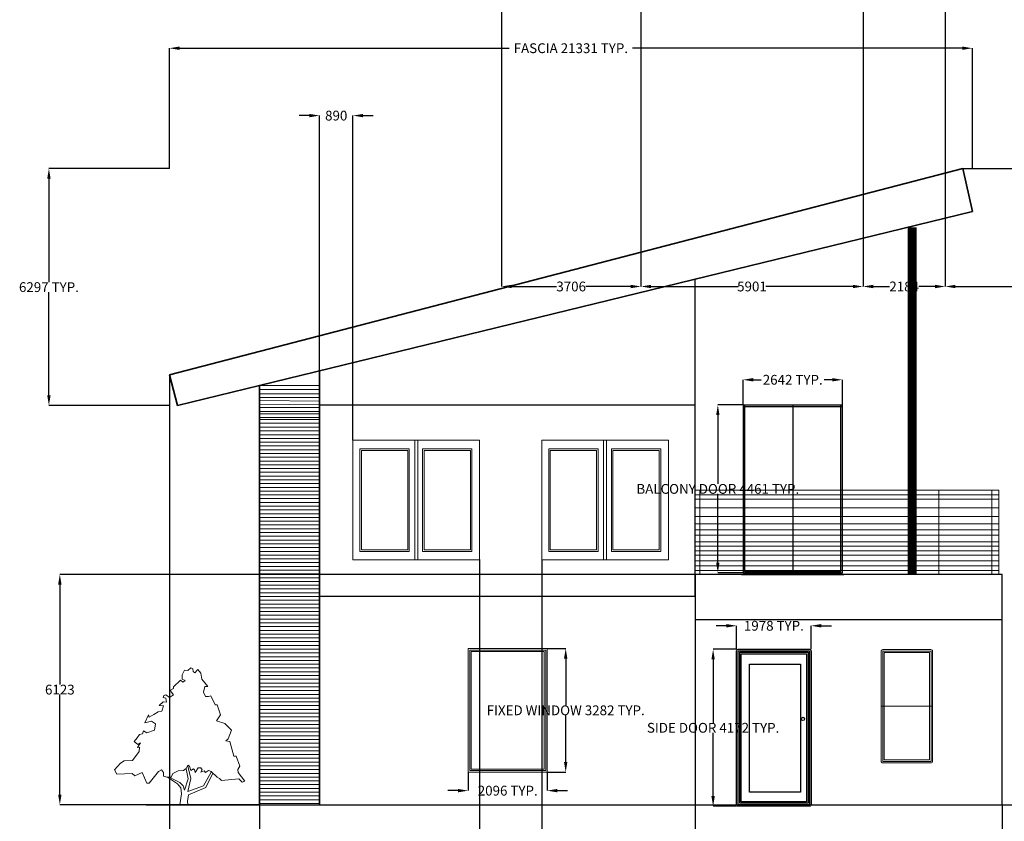
# Model space of a CAD drawing. Units: millimetres. Extents: x 23 to 3809233, y 4 to 290343.
# Tile 4 of 8: x 1889493 to 1915648, y 151826 to 173128. Entities that reach past the tile are written whole.
import ezdxf

# ---------------------------------------------------------------- set-up
doc = ezdxf.new("R2010")
doc.units = ezdxf.units.MM
doc.header["$MEASUREMENT"] = 0
for name, color, linetype, lineweight in [('A-ANNO-DIMS', 2, 'Continuous', 18), ('A-COLS', 7, 'Continuous', 35), ('A-DOOR', 3, 'Continuous', 25), ('A-ELEV', 7, 'Continuous', 25), ('A-ELEV-GRND', 7, 'Continuous', 30), ('A-FLOR-RAIL', 8, 'Continuous', 18), ('A-GLAZ', 4, 'Continuous', 18), ('A-ROOF', 7, 'Continuous', 35), ('A-WALL-PATT', 252, 'Continuous', 13), ('L-PLNT', 94, 'Continuous', 13)]:
    doc.layers.add(name, color=color, linetype=linetype, lineweight=lineweight)
doc.styles.get("Standard").update_dxf_attribs({"font": 'arial.ttf'})
doc.dimstyles.get("Standard").update_dxf_attribs({"dimtxt": 260.18, "dimasz": 270.18, "dimexe": 0.18, "dimexo": 0.0625, "dimgap": 0.09, "dimtad": 0, "dimtih": 1, "dimtoh": 1, "dimdec": 0, "dimzin": 0, "dimdsep": 46, "dimtxsty": 'Standard', "dimcen": 0.09, "dimadec": 0, "dimazin": 0, "dimtfac": 1, "dimtdec": 0, "dimtofl": 0, "dimtmove": 0, "dimatfit": 3, "dimfxl": 1, "dimtolj": 1, "dimtzin": 0, "dimarcsym": 0})

# ---------------------------------------------------------------- blocks, each defined once
blk = doc.blocks.new('*U4')
for points in [[(22.0124, 137.721), (18.5475, 141.5624), (15.5282, 138.2446), (13.8028, 139.3505), (13.3714, 142.1153), (11.2148, 143.2214), (8.1954, 140.4564), (4.7447, 141.0094), (2.1567, 136.0326), (2.1567, 131.6088), (5.6074, 129.9499), (3.0193, 128.2909), (0.4313, 130.5029), (-6.9015, 123.3141), (-6.9015, 121.6552), (-9.9208, 119.9963), (-9.0581, 118.3373), (-6.9015, 115.0195), (-10.7835, 112.2546), (-14.6656, 115.0195), (-16.8222, 114.4665), (-17.6849, 112.2546), (-14.6656, 111.7016), (-14.2342, 107.2778), (-17.6065, 107.8307), (-21.5669, 103.9599), (-17.2536, 103.4069), (-18.9789, 97.8771), (-22.8609, 97.3241), (-27.1743, 94.5593), (-32.3504, 91.7944), (-32.7817, 94.0063), (-36.6638, 85.7116), (-29.7624, 87.3705), (-25.449, 84.6056), (-26.743, 77.9699), (-34.507, 75.205), (-37.9578, 77.4169), (-39.2518, 74.099), (-42.2711, 73.5461), (-44.8592, 70.2282), (-47.8786, 66.3574), (-43.9965, 63.0395), (-41.4085, 64.6985), (-44.3346, 59.8898), (-42.2089, 60.1377), (-42.5159, 55.7849), (-49.6039, 46.4502), (-58.2307, 45.8972), (-62.1127, 43.6853), (-68.5828, 36.4966), (-65.9947, 32.0727), (-50.0352, 32.6257), (-47.0159, 30.4138), (-39.6831, 33.7317), (-34.507, 22.6721), (-32.3504, 22.6721), (-22.4296, 34.8376), (-19.4102, 36.4966), (-17.2536, 33.7317), (-17.2536, 29.8608), (-13.8028, 28.7549), (-9.0581, 28.7549), (-7.3328, 32.6257), (-1.7254, 35.3906), (3.8821, 35.9436), (6.4701, 38.1555), (6.9014, 38.7085), (8.1954, 41.4734), (9.9208, 40.3674), (11.2148, 35.9436), (14.2341, 37.6025), (15.0968, 36.4966), (15.9595, 33.7317), (18.9789, 38.7085), (21.9982, 38.7085), (23.2922, 36.4966), (21.9982, 34.2847), (25.4489, 35.3906), (26.743, 33.7317), (29.7623, 35.9436), (32.7817, 34.8376), (38.8204, 28.7549), (41.4084, 27.6489), (43.5651, 25.437), (61.6813, 27.0959), (65.132, 23.7781), (67.7201, 24.884), (60.8186, 33.7317), (60.3873, 37.0495), (62.544, 40.3674), (58.662, 50.874), (56.5053, 50.874), (52.1919, 66.3574), (47.8785, 66.9103), (50.4665, 69.1222), (53.9172, 77.9699), (47.0158, 85.1586), (38.3891, 87.9235), (42.2711, 94.0063)], [(42.2711, 94.0063), (38.8204, 104.5129), (36.6637, 104.5129), (32.3503, 113.9135), (29.7623, 113.3605), (26.743, 113.3605), (24.5862, 117.7844), (25.8802, 123.8671), (29.331, 123.8671), (22.8609, 131.6088), (21.9982, 137.6916)], [(-9.9208, 28.2019), (0, 23.2251), (3.4507, 19.9072), (4.7447, 15.4834), (8.6267, 27.0959), (6.4701, 37.6025)], [(34.5071, 33.1787), (27.1743, 18.2483), (9.0581, 10.5066), (7.7641, 3.8708), (8.1954, 0)], [(8.1954, 40.3674), (11.2148, 27.6489), (8.1954, 13.8245), (24.5862, 19.9072), (32.7817, 34.2847)], [(-12.9401, 28.7549), (-2.588, 22.1191), (0.8626, 17.6953), (1.7253, 11.6125), (0, 0)]]:
    blk.add_lwpolyline(points)
blk = doc.blocks.new('SIDE-ENTRY-DOOR-ELEV')
for points in [[(0, 4129, -0.414214), (43, 4172), (1935, 4172, -0.414214), (1978, 4129), (1978, 43, -0.414214), (1935, 0), (43, 0, -0.414214), (0, 43)], [(40, 4129, -0.414214), (43, 4132), (1935, 4132, -0.414214), (1938, 4129), (1938, 43, -0.414214), (1935, 40), (43, 40, -0.414214), (40, 43)], [(337, 3772, -0.414214), (340, 3775), (1691, 3775, -0.414214), (1694, 3772), (1694, 380, -0.414214), (1691, 377), (340, 377, -0.414214), (337, 380)]]:
    blk.add_lwpolyline(points, format="xyb", close=True)
for points in [[(80, 4092), (1898, 4092), (1898, 80), (80, 80)], [(120, 4052), (1858, 4052), (1858, 120), (120, 120)]]:
    blk.add_lwpolyline(points, close=True)
blk.add_circle((1762, 2322), 43.3)
blk = doc.blocks.new('FIXED-WINDOW-ELEV')
blk.add_lwpolyline([(0, 3279, -0.414214), (3, 3282), (2093, 3282, -0.414214), (2096, 3279), (2096, 3, -0.414214), (2093, 0), (3, 0, -0.414214), (0, 3)], format="xyb", close=True)
for points in [[(40, 3242), (2056, 3242), (2056, 40), (40, 40)], [(80, 3202), (2016, 3202), (2016, 80), (80, 80)]]:
    blk.add_lwpolyline(points, close=True)
blk = doc.blocks.new('TRANSOM-WINDOW-ELEV')
blk.add_line((0, 1506), (1365, 1506))
for points in [[(0, 2969, -0.414214), (43, 3012), (1322, 3012, -0.414214), (1365, 2969), (1365, 43, -0.414214), (1322, 0), (43, 0, -0.414214), (0, 43)], [(40, 2969, -0.414214), (43, 2972), (1322, 2972, -0.414214), (1325, 2969), (1325, 43, -0.414214), (1322, 40), (43, 40, -0.414214), (40, 43)]]:
    blk.add_lwpolyline(points, format="xyb", close=True)
blk.add_lwpolyline([(80, 2932), (1285, 2932), (1285, 80), (80, 80)], close=True)
blk = doc.blocks.new('BALCONY-GUARD-ELEV')
for p, q in [((8065, 2239), (0, 2239)), ((0, 2109), (8065, 2109)), ((129, 2239), (129, 0)), ((6472, 2239), (6472, 0)), ((7879, 2239), (7879, 0)), ((8065, 0), (8065, 2239)), ((0, 1995), (8065, 1995)), ((0, 1772), (8065, 1772)), ((0, 1540), (8065, 1540)), ((0, 1341), (8065, 1341)), ((0, 1187), (8065, 1187)), ((0, 1045), (8065, 1045)), ((0, 866), (8065, 866)), ((0, 745), (8065, 745)), ((0, 622), (8065, 622)), ((0, 507), (8065, 507)), ((0, 360), (8065, 360)), ((8065, 360), (8065, 360)), ((0, 225), (8065, 225)), ((0, 103), (8065, 103))]:
    blk.add_line(p, q)
blk = doc.blocks.new('ROOF-FASCIA-SIDE-ELEV')
for p, q in [((21076, 6297), (0, 817)), ((21331, 5154), (21076, 6297)), ((2399, 534), (21331, 5154)), ((0, 817), (212, 0)), ((2399, 534), (212, 0))]:
    blk.add_line(p, q)
blk = doc.blocks.new('BALCONY-SUPPORT-ELEV')
for p, q in [((0, 0), (0, 9216)), ((40, 0), (40, 9216)), ((80, 0), (80, 9216)), ((120, 0), (120, 9216)), ((120, 0), (120, 9216)), ((160, 0), (160, 9216)), ((200, 0), (200, 9216))]:
    blk.add_line(p, q)
blk = doc.blocks.new('BALCONY-GLAZED-DOOR-ELEV')
for p, q in [((0, 4461), (2642, 4461)), ((1321, 4461), (1321, 0)), ((0, 4421), (2642, 4421))]:
    blk.add_line(p, q)
for points in [[(0, 4461), (0, 0), (2642, 0), (2642, 4461)], [(40, 4461), (40, 40), (2602, 40), (2602, 4461)]]:
    blk.add_lwpolyline(points)
blk = doc.blocks.new('*D28')
at = {"layer": 'A-ANNO-DIMS', "color": 0, "lineweight": -2, "transparency": 16777216}
for p, q in [((1893468, 169170), (1893468, 172370)), ((1893739, 172370), (1902498, 172370)), ((1914529, 172370), (1905770, 172370)), ((1914799, 169170), (1914799, 172370))]:
    blk.add_line(p, q, dxfattribs=at)
at = {"layer": 'A-ANNO-DIMS', "color": 0, "transparency": 16777216}
for points in [[(1893739, 172415), (1893739, 172325), (1893468, 172370)], [(1914529, 172415), (1914529, 172325), (1914799, 172370)]]:
    blk.add_solid(points, dxfattribs=at)
at = {"layer": 'Defpoints', "color": 0, "transparency": 16777216}
for p in [(1914799, 172370), (1893468, 169170), (1914799, 169170)]:
    blk.add_point(p, dxfattribs=at)
at = {"layer": 'A-ANNO-DIMS', "color": 0, "transparency": 16777216, "insert": (1904134, 172370), "char_height": 260.18, "attachment_point": 5}
blk.add_mtext('\\A1;FASCIA 21331 TYP.', dxfattribs=at)
blk = doc.blocks.new('*D29')
at = {"layer": 'A-ANNO-DIMS', "color": 0, "lineweight": -2, "transparency": 16777216}
for p, q in [((1893468, 169170), (1890268, 169170)), ((1890269, 168900), (1890269, 166154)), ((1890269, 163143), (1890269, 165889)), ((1893468, 162873), (1890268, 162873))]:
    blk.add_line(p, q, dxfattribs=at)
at = {"layer": 'A-ANNO-DIMS', "color": 0, "transparency": 16777216}
for points in [[(1890224, 168900), (1890314, 168900), (1890269, 169170)], [(1890224, 163143), (1890314, 163143), (1890269, 162873)]]:
    blk.add_solid(points, dxfattribs=at)
at = {"layer": 'Defpoints', "color": 0, "transparency": 16777216}
for p in [(1890269, 169170), (1893468, 169170), (1893468, 162873)]:
    blk.add_point(p, dxfattribs=at)
at = {"layer": 'A-ANNO-DIMS', "color": 0, "transparency": 16777216, "insert": (1890269, 166021), "char_height": 260.18, "attachment_point": 5}
blk.add_mtext('\\A1;6297 TYP.', dxfattribs=at)
blk = doc.blocks.new('*D32')
at = {"layer": 'A-ANNO-DIMS', "color": 0, "lineweight": -2, "transparency": 16777216}
for p, q in [((1908707, 162890), (1908038, 162890)), ((1908038, 162620), (1908038, 160794)), ((1908038, 158699), (1908038, 160524)), ((1908707, 158429), (1908038, 158429))]:
    blk.add_line(p, q, dxfattribs=at)
at = {"layer": 'A-ANNO-DIMS', "color": 0, "transparency": 16777216}
for points in [[(1907993, 162620), (1908083, 162620), (1908038, 162890)], [(1907993, 158699), (1908083, 158699), (1908038, 158429)]]:
    blk.add_solid(points, dxfattribs=at)
at = {"layer": 'Defpoints', "color": 0, "transparency": 16777216}
for p in [(1908038, 162890), (1908707, 162890), (1908707, 158429)]:
    blk.add_point(p, dxfattribs=at)
at = {"layer": 'A-ANNO-DIMS', "color": 0, "transparency": 16777216, "insert": (1908038, 160659), "char_height": 260.18, "attachment_point": 5}
blk.add_mtext('\\A1;BALCONY DOOR 4461 TYP.', dxfattribs=at)
blk = doc.blocks.new('*D33')
at = {"layer": 'A-ANNO-DIMS', "color": 0, "lineweight": -2, "transparency": 16777216}
for p, q in [((1908707, 162890), (1908707, 163559)), ((1908977, 163559), (1909190, 163559)), ((1911079, 163559), (1910866, 163559)), ((1911349, 162890), (1911349, 163559))]:
    blk.add_line(p, q, dxfattribs=at)
at = {"layer": 'A-ANNO-DIMS', "color": 0, "transparency": 16777216}
for points in [[(1908977, 163604), (1908977, 163514), (1908707, 163559)], [(1911079, 163604), (1911079, 163514), (1911349, 163559)]]:
    blk.add_solid(points, dxfattribs=at)
at = {"layer": 'Defpoints', "color": 0, "transparency": 16777216}
for p in [(1911349, 163559), (1908707, 162890), (1911349, 162890)]:
    blk.add_point(p, dxfattribs=at)
at = {"layer": 'A-ANNO-DIMS', "color": 0, "transparency": 16777216, "insert": (1910028, 163559), "char_height": 260.18, "attachment_point": 5}
blk.add_mtext('\\A1;2642 TYP.', dxfattribs=at)
blk = doc.blocks.new('*D34')
at = {"layer": 'A-ANNO-DIMS', "color": 0, "lineweight": -2, "transparency": 16777216}
for p, q in [((1908538, 156397), (1907912, 156397)), ((1907913, 156126), (1907913, 154445)), ((1907913, 152495), (1907913, 154176)), ((1908538, 152225), (1907912, 152225))]:
    blk.add_line(p, q, dxfattribs=at)
at = {"layer": 'A-ANNO-DIMS', "color": 0, "transparency": 16777216}
for points in [[(1907868, 156126), (1907958, 156126), (1907913, 156397)], [(1907868, 152495), (1907958, 152495), (1907913, 152225)]]:
    blk.add_solid(points, dxfattribs=at)
at = {"layer": 'Defpoints', "color": 0, "transparency": 16777216}
for p in [(1907913, 156397), (1908538, 156397), (1908538, 152225)]:
    blk.add_point(p, dxfattribs=at)
at = {"layer": 'A-ANNO-DIMS', "color": 0, "transparency": 16777216, "insert": (1907913, 154311), "char_height": 260.18, "attachment_point": 5}
blk.add_mtext('\\A1;SIDE DOOR 4172 TYP.', dxfattribs=at)
blk = doc.blocks.new('*D35')
at = {"layer": 'A-ANNO-DIMS', "color": 0, "lineweight": -2, "transparency": 16777216}
for p, q in [((1908268, 157022), (1907998, 157022)), ((1908538, 156397), (1908538, 157023)), ((1910516, 156397), (1910516, 157023)), ((1910786, 157022), (1911056, 157022))]:
    blk.add_line(p, q, dxfattribs=at)
at = {"layer": 'A-ANNO-DIMS', "color": 0, "transparency": 16777216}
for points in [[(1908268, 157067), (1908268, 156977), (1908538, 157022)], [(1910786, 157067), (1910786, 156977), (1910516, 157022)]]:
    blk.add_solid(points, dxfattribs=at)
at = {"layer": 'Defpoints', "color": 0, "transparency": 16777216}
for p in [(1910516, 157022), (1908538, 156397), (1910516, 156397)]:
    blk.add_point(p, dxfattribs=at)
at = {"layer": 'A-ANNO-DIMS', "color": 0, "transparency": 16777216, "insert": (1909527, 157022), "char_height": 260.18, "attachment_point": 5}
blk.add_mtext('\\A1;1978 TYP.', dxfattribs=at)
blk = doc.blocks.new('*D36')
at = {"layer": 'A-ANNO-DIMS', "color": 0, "lineweight": -2, "transparency": 16777216}
for p, q in [((1903505, 156416), (1903997, 156416)), ((1903997, 156146), (1903997, 154910)), ((1903997, 153404), (1903997, 154640)), ((1903505, 153134), (1903997, 153134))]:
    blk.add_line(p, q, dxfattribs=at)
at = {"layer": 'A-ANNO-DIMS', "color": 0, "transparency": 16777216}
for points in [[(1903952, 156146), (1904042, 156146), (1903997, 156416)], [(1903952, 153404), (1904042, 153404), (1903997, 153134)]]:
    blk.add_solid(points, dxfattribs=at)
at = {"layer": 'Defpoints', "color": 0, "transparency": 16777216}
for p in [(1903505, 156416), (1903997, 156416), (1903505, 153134)]:
    blk.add_point(p, dxfattribs=at)
at = {"layer": 'A-ANNO-DIMS', "color": 0, "transparency": 16777216, "insert": (1903997, 154775), "char_height": 260.18, "attachment_point": 5}
blk.add_mtext('\\A1;FIXED WINDOW 3282 TYP.', dxfattribs=at)
blk = doc.blocks.new('*D37')
at = {"layer": 'A-ANNO-DIMS', "color": 0, "lineweight": -2, "transparency": 16777216}
for p, q in [((1901409, 153134), (1901409, 152641)), ((1903505, 153134), (1903505, 152641)), ((1901139, 152641), (1900869, 152641)), ((1903775, 152641), (1904045, 152641))]:
    blk.add_line(p, q, dxfattribs=at)
at = {"layer": 'A-ANNO-DIMS', "color": 0, "transparency": 16777216}
for points in [[(1901139, 152686), (1901139, 152596), (1901409, 152641)], [(1903775, 152686), (1903775, 152596), (1903505, 152641)]]:
    blk.add_solid(points, dxfattribs=at)
at = {"layer": 'Defpoints', "color": 0, "transparency": 16777216}
for p in [(1901409, 153134), (1903505, 153134), (1903505, 152641)]:
    blk.add_point(p, dxfattribs=at)
at = {"layer": 'A-ANNO-DIMS', "color": 0, "transparency": 16777216, "insert": (1902457, 152641), "char_height": 260.18, "attachment_point": 5}
blk.add_mtext('\\A1;2096 TYP.', dxfattribs=at)
blk = doc.blocks.new('*D80')
at = {"layer": 'A-ANNO-DIMS', "color": 0, "lineweight": -2, "transparency": 16777216}
for p, q in [((1893468, 163690), (1893468, 149029)), ((1915588, 152264), (1915588, 149029)), ((1893739, 149029), (1904037, 149029)), ((1915318, 149029), (1905020, 149029))]:
    blk.add_line(p, q, dxfattribs=at)
at = {"layer": 'A-ANNO-DIMS', "color": 0, "transparency": 16777216}
for points in [[(1893739, 149074), (1893739, 148984), (1893468, 149029)], [(1915318, 149074), (1915318, 148984), (1915588, 149029)]]:
    blk.add_solid(points, dxfattribs=at)
at = {"layer": 'Defpoints', "color": 0, "transparency": 16777216}
for p in [(1893468, 163690), (1915588, 152265), (1915588, 149029)]:
    blk.add_point(p, dxfattribs=at)
at = {"layer": 'A-ANNO-DIMS', "color": 0, "transparency": 16777216, "insert": (1904528, 149029), "char_height": 260.2, "attachment_point": 5}
blk.add_mtext('\\A1;22120', dxfattribs=at)
blk = doc.blocks.new('*D81')
at = {"layer": 'A-ANNO-DIMS', "color": 0, "lineweight": -2, "transparency": 16777216}
for p, q in [((1914545, 169170), (1921388, 169170)), ((1921387, 168900), (1921387, 160850)), ((1921387, 152535), (1921387, 160584)), ((1915588, 152265), (1921388, 152265))]:
    blk.add_line(p, q, dxfattribs=at)
at = {"layer": 'A-ANNO-DIMS', "color": 0, "transparency": 16777216}
for points in [[(1921342, 168900), (1921433, 168900), (1921387, 169170)], [(1921342, 152535), (1921433, 152535), (1921387, 152265)]]:
    blk.add_solid(points, dxfattribs=at)
at = {"layer": 'Defpoints', "color": 0, "transparency": 16777216}
for p in [(1914545, 169170), (1921387, 169170), (1915588, 152265)]:
    blk.add_point(p, dxfattribs=at)
at = {"layer": 'A-ANNO-DIMS', "color": 0, "transparency": 16777216, "insert": (1921387, 160717), "char_height": 260.2, "attachment_point": 5}
blk.add_mtext('\\A1;16905', dxfattribs=at)
blk = doc.blocks.new('*D82')
at = {"layer": 'A-ANNO-DIMS', "color": 0, "lineweight": -2, "transparency": 16777216}
for p, q in [((1895867, 152264), (1895867, 149029)), ((1907434, 152264), (1907434, 149029)), ((1896137, 149029), (1901173, 149029)), ((1907164, 149029), (1902128, 149029))]:
    blk.add_line(p, q, dxfattribs=at)
at = {"layer": 'A-ANNO-DIMS', "color": 0, "transparency": 16777216}
for points in [[(1896137, 149074), (1896137, 148984), (1895867, 149029)], [(1907164, 149074), (1907164, 148984), (1907434, 149029)]]:
    blk.add_solid(points, dxfattribs=at)
at = {"layer": 'Defpoints', "color": 0, "transparency": 16777216}
for p in [(1895867, 152265), (1907434, 152265), (1907434, 149029)]:
    blk.add_point(p, dxfattribs=at)
at = {"layer": 'A-ANNO-DIMS', "color": 0, "transparency": 16777216, "insert": (1901651, 149029), "char_height": 260.2, "attachment_point": 5}
blk.add_mtext('\\A1;11567', dxfattribs=at)
blk = doc.blocks.new('*D83')
at = {"layer": 'A-ANNO-DIMS', "color": 0, "lineweight": -2, "transparency": 16777216}
for p, q in [((1907435, 158388), (1890558, 158388)), ((1890559, 158117), (1890559, 155459)), ((1890559, 152535), (1890559, 155193)), ((1895867, 152265), (1890558, 152265))]:
    blk.add_line(p, q, dxfattribs=at)
at = {"layer": 'A-ANNO-DIMS', "color": 0, "transparency": 16777216}
for points in [[(1890514, 158117), (1890604, 158117), (1890559, 158388)], [(1890514, 152535), (1890604, 152535), (1890559, 152265)]]:
    blk.add_solid(points, dxfattribs=at)
at = {"layer": 'Defpoints', "color": 0, "transparency": 16777216}
for p in [(1890559, 158388), (1907435, 158388), (1895867, 152265)]:
    blk.add_point(p, dxfattribs=at)
at = {"layer": 'A-ANNO-DIMS', "color": 0, "transparency": 16777216, "insert": (1890559, 155326), "char_height": 260.2, "attachment_point": 5}
blk.add_mtext('\\A1;6123', dxfattribs=at)
blk = doc.blocks.new('*D84')
at = {"layer": 'A-ANNO-DIMS', "color": 0, "lineweight": -2, "transparency": 16777216}
for p, q in [((1897185, 170579), (1896915, 170579)), ((1897456, 162891), (1897456, 170580)), ((1898346, 161958), (1898346, 170580)), ((1898616, 170579), (1898886, 170579))]:
    blk.add_line(p, q, dxfattribs=at)
at = {"layer": 'A-ANNO-DIMS', "color": 0, "transparency": 16777216}
for points in [[(1897185, 170624), (1897185, 170534), (1897456, 170579)], [(1898616, 170624), (1898616, 170534), (1898346, 170579)]]:
    blk.add_solid(points, dxfattribs=at)
at = {"layer": 'Defpoints', "color": 0, "transparency": 16777216}
for p in [(1898346, 170579), (1897456, 162891), (1898346, 161958)]:
    blk.add_point(p, dxfattribs=at)
at = {"layer": 'A-ANNO-DIMS', "color": 0, "transparency": 16777216, "insert": (1897901, 170579), "char_height": 260.2, "attachment_point": 5}
blk.add_mtext('\\A1;890', dxfattribs=at)
blk = doc.blocks.new('*D85')
at = {"layer": 'A-ANNO-DIMS', "color": 0, "lineweight": -2, "transparency": 16777216}
for p, q in [((1901710, 158781), (1901710, 149029)), ((1903361, 158781), (1903361, 149029)), ((1901980, 149029), (1902184, 149029)), ((1903091, 149029), (1902887, 149029))]:
    blk.add_line(p, q, dxfattribs=at)
at = {"layer": 'A-ANNO-DIMS', "color": 0, "transparency": 16777216}
for points in [[(1901980, 149074), (1901980, 148984), (1901710, 149029)], [(1903091, 149074), (1903091, 148984), (1903361, 149029)]]:
    blk.add_solid(points, dxfattribs=at)
at = {"layer": 'Defpoints', "color": 0, "transparency": 16777216}
for p in [(1901710, 158781), (1903361, 158781), (1903361, 149029)]:
    blk.add_point(p, dxfattribs=at)
at = {"layer": 'A-ANNO-DIMS', "color": 0, "transparency": 16777216, "insert": (1902536, 149029), "char_height": 260.2, "attachment_point": 5}
blk.add_mtext('\\A1;1651', dxfattribs=at)
blk = doc.blocks.new('*D96')
at = {"layer": 'A-ANNO-DIMS', "color": 0, "lineweight": -2, "transparency": 16777216}
for p, q in [((1902289, 175032), (1902289, 166038)), ((1905995, 175031), (1905995, 166038)), ((1902560, 166038), (1903754, 166038)), ((1905725, 166038), (1904531, 166038))]:
    blk.add_line(p, q, dxfattribs=at)
at = {"layer": 'A-ANNO-DIMS', "color": 0, "transparency": 16777216}
for points in [[(1902560, 166083), (1902560, 165993), (1902289, 166038)], [(1905725, 166083), (1905725, 165993), (1905995, 166038)]]:
    blk.add_solid(points, dxfattribs=at)
at = {"layer": 'Defpoints', "color": 0, "transparency": 16777216}
for p in [(1902289, 175032), (1905995, 175031), (1905995, 166038)]:
    blk.add_point(p, dxfattribs=at)
at = {"layer": 'A-ANNO-DIMS', "color": 0, "transparency": 16777216, "insert": (1904142, 166038), "char_height": 260.2, "attachment_point": 5}
blk.add_mtext('\\A1;3706', dxfattribs=at)
blk = doc.blocks.new('*D97')
at = {"layer": 'A-ANNO-DIMS', "color": 0, "lineweight": -2, "transparency": 16777216}
for p, q in [((1905995, 175031), (1905995, 166038)), ((1911896, 175048), (1911896, 166038)), ((1906265, 166038), (1908582, 166038)), ((1911626, 166038), (1909309, 166038))]:
    blk.add_line(p, q, dxfattribs=at)
at = {"layer": 'A-ANNO-DIMS', "color": 0, "transparency": 16777216}
for points in [[(1906265, 166083), (1906265, 165993), (1905995, 166038)], [(1911626, 166083), (1911626, 165993), (1911896, 166038)]]:
    blk.add_solid(points, dxfattribs=at)
at = {"layer": 'Defpoints', "color": 0, "transparency": 16777216}
for p in [(1905995, 175031), (1911896, 175048), (1911896, 166038)]:
    blk.add_point(p, dxfattribs=at)
at = {"layer": 'A-ANNO-DIMS', "color": 0, "transparency": 16777216, "insert": (1908945, 166038), "char_height": 260.2, "attachment_point": 5}
blk.add_mtext('\\A1;5901', dxfattribs=at)
blk = doc.blocks.new('*D98')
at = {"layer": 'A-ANNO-DIMS', "color": 0, "lineweight": -2, "transparency": 16777216}
for p, q in [((1911896, 175048), (1911896, 166038)), ((1914080, 175026), (1914080, 166038)), ((1912166, 166038), (1912598, 166038)), ((1913810, 166038), (1913378, 166038))]:
    blk.add_line(p, q, dxfattribs=at)
at = {"layer": 'A-ANNO-DIMS', "color": 0, "transparency": 16777216}
for points in [[(1912166, 166083), (1912166, 165993), (1911896, 166038)], [(1913810, 166083), (1913810, 165993), (1914080, 166038)]]:
    blk.add_solid(points, dxfattribs=at)
at = {"layer": 'Defpoints', "color": 0, "transparency": 16777216}
for p in [(1911896, 175048), (1914080, 175026), (1914080, 166038)]:
    blk.add_point(p, dxfattribs=at)
at = {"layer": 'A-ANNO-DIMS', "color": 0, "transparency": 16777216, "insert": (1912988, 166038), "char_height": 260.2, "attachment_point": 5}
blk.add_mtext('\\A1;2184', dxfattribs=at)
blk = doc.blocks.new('*D102')
at = {"layer": 'A-ANNO-DIMS', "color": 0, "lineweight": -2, "transparency": 16777216}
for p, q in [((1914079.851314, 175025.824019), (1914079.851314, 166037.51032)), ((1921856.95103, 175025.824019), (1921856.95103, 166037.51032)), ((1914350.031314, 166037.69032), (1917580.88079, 166037.69032)), ((1921586.77103, 166037.69032), (1918355.921554, 166037.69032))]:
    blk.add_line(p, q, dxfattribs=at)
at = {"layer": 'A-ANNO-DIMS', "color": 0, "transparency": 16777216}
for points in [[(1914350.031314, 166082.72032), (1914350.031314, 165992.66032), (1914079.851314, 166037.69032)], [(1921586.77103, 166082.72032), (1921586.77103, 165992.66032), (1921856.95103, 166037.69032)]]:
    blk.add_solid(points, dxfattribs=at)
at = {"layer": 'Defpoints', "color": 0, "transparency": 16777216}
for p in [(1914079.851314, 175025.886519), (1921856.95103, 175025.886519), (1921856.95103, 166037.69032)]:
    blk.add_point(p, dxfattribs=at)
at = {"layer": 'A-ANNO-DIMS', "color": 0, "transparency": 16777216, "insert": (1917968.401172, 166037.69032), "char_height": 260.18, "attachment_point": 5}
blk.add_mtext('\\A1;7777', dxfattribs=at)

msp = doc.modelspace()

# ---------------------------------------------------------------- hatches: boundary and pattern name
at = {"layer": 'A-WALL-PATT'}
h = msp.add_hatch(dxfattribs=at)
h.set_pattern_fill('ANSI31', color=256, scale=800, angle=-45, style=0)
h.paths.add_polyline_path([(1895867.197, 152264.531), (1897455.656, 152264.531), (1897455.656, 162369.95), (1895867.197, 162369.95)])

# ---------------------------------------------------------------- linework, layer by layer
at = {"layer": 'A-COLS'}
for p, q in [((1897455.656, 152264.531), (1897455.656, 163794.299)), ((1895867.197, 152264.531), (1895867.197, 163406.613))]:
    msp.add_line(p, q, dxfattribs=at)
at = {"layer": 'A-DOOR'}
msp.add_lwpolyline([(1908666.946, 158391.548, 0.414213562), (1908669.946, 158388.548), (1911385.771, 158388.548, 0.414213562), (1911388.771, 158391.548)], format="xyb", dxfattribs=at)
at = {"layer": 'A-ELEV'}
for p, q in [((1907434.445, 157807.695), (1907434.445, 166229.765)), ((1897455.656, 162891.03), (1907434.445, 162891.03)), ((1915588.32, 152264.531), (1915588.32, 158385.548)), ((1897455.656, 157807.695), (1907434.445, 157807.695)), ((1907434.445, 157807.695), (1907434.445, 152264.531))]:
    msp.add_line(p, q, dxfattribs=at)
msp.add_lwpolyline([(1907434.445, 157192.635, 0.414213562), (1907437.445, 157189.635), (1915585.32, 157189.635, 0.414213562), (1915588.32, 157192.635), (1915588.32, 158385.548, 0.414213562), (1915585.32, 158388.548), (1907437.445, 158388.548, 0.414213562), (1907434.445, 158385.548)], format="xyb", close=True, dxfattribs=at)
at = {"layer": 'A-ELEV-GRND'}
msp.add_line((1892849.81, 152264.531), (1919977.977, 152264.531), dxfattribs=at)
at = {"layer": 'A-GLAZ'}
for p, q in [((1899986.953, 161958.11), (1899986.953, 158777.768)), ((1900066.953, 161958.11), (1900066.953, 158777.768)), ((1905004.216, 161958.11), (1905004.216, 158777.768)), ((1905084.216, 161958.11), (1905084.216, 158777.768))]:
    msp.add_line(p, q, dxfattribs=at)
for points in [[(1898343.83, 161955.11, -0.414213562), (1898346.83, 161958.11), (1901707.076, 161958.11, -0.414213562), (1901710.076, 161955.11), (1901710.076, 158780.768, -0.414213562), (1901707.076, 158777.768), (1898346.83, 158777.768, -0.414213562), (1898343.83, 158780.768)], [(1903361.093, 161955.11, -0.414213562), (1903364.093, 161958.11), (1906724.34, 161958.11, -0.414213562), (1906727.34, 161955.11), (1906727.34, 158780.768, -0.414213562), (1906724.34, 158777.768), (1903364.093, 158777.768, -0.414213562), (1903361.093, 158780.768)], [(1898529.191, 161720.123, -0.414213562), (1898532.191, 161723.123), (1899837.574, 161723.123, -0.414213562), (1899840.574, 161720.123), (1899840.574, 158999.449, -0.414213562), (1899837.574, 158996.449), (1898532.191, 158996.449, -0.414213562), (1898529.191, 158999.449)], [(1900195.226, 161720.123, -0.414213562), (1900198.226, 161723.123), (1901503.608, 161723.123, -0.414213562), (1901506.608, 161720.123), (1901506.608, 158999.449, -0.414213562), (1901503.608, 158996.449), (1900198.226, 158996.449, -0.414213562), (1900195.226, 158999.449)], [(1903546.454, 161720.123, -0.414213562), (1903549.454, 161723.123), (1904854.837, 161723.123, -0.414213562), (1904857.837, 161720.123), (1904857.837, 158999.449, -0.414213562), (1904854.837, 158996.449), (1903549.454, 158996.449, -0.414213562), (1903546.454, 158999.449)], [(1905212.489, 161720.123, -0.414213562), (1905215.489, 161723.123), (1906520.872, 161723.123, -0.414213562), (1906523.872, 161720.123), (1906523.872, 158999.449, -0.414213562), (1906520.872, 158996.449), (1905215.489, 158996.449, -0.414213562), (1905212.489, 158999.449)]]:
    msp.add_lwpolyline(points, format="xyb", close=True, dxfattribs=at)
for points in [[(1898569.191, 161683.123), (1899800.574, 161683.123), (1899800.574, 159036.449), (1898569.191, 159036.449)], [(1900235.226, 161683.123), (1901466.608, 161683.123), (1901466.608, 159036.449), (1900235.226, 159036.449)], [(1903586.454, 161683.123), (1904817.837, 161683.123), (1904817.837, 159036.449), (1903586.454, 159036.449)], [(1905252.489, 161683.123), (1906483.872, 161683.123), (1906483.872, 159036.449), (1905252.489, 159036.449)]]:
    msp.add_lwpolyline(points, close=True, dxfattribs=at)
at = {"layer": 'A-WALL-PATT'}
for p, q in [((1895867.197, 163404.159), (1897455.656, 163404.159)), ((1895867.197, 163304.159), (1897455.656, 163304.159)), ((1895867.197, 163189.007), (1897455.656, 163189.007)), ((1895867.197, 163089.007), (1897455.656, 163089.007)), ((1895868.541, 163012.38), (1897457.001, 162991.021)), ((1895867.197, 162912.389), (1897455.656, 162891.03)), ((1895867.197, 162820.23), (1897455.656, 162820.23)), ((1895867.197, 162720.23), (1897455.656, 162720.23)), ((1895867.197, 162657.251), (1897455.656, 162657.251)), ((1895867.197, 162557.251), (1897455.656, 162557.251)), ((1895867.197, 162502.159), (1897455.656, 162502.159)), ((1895867.197, 162402.159), (1897455.656, 162402.159))]:
    msp.add_line(p, q, dxfattribs=at)

# ---------------------------------------------------------------- block references
at = {"layer": 'A-COLS'}
msp.add_blockref('BALCONY-SUPPORT-ELEV', (1913101.362, 158388.548), dxfattribs=at)
at = {"layer": 'A-DOOR'}
for name, p in [('BALCONY-GLAZED-DOOR-ELEV', (1908706.946, 158428.548)), ('SIDE-ENTRY-DOOR-ELEV', (1908538.443, 152224.531))]:
    msp.add_blockref(name, p, dxfattribs=at)
at = {"layer": 'A-FLOR-RAIL'}
msp.add_blockref('BALCONY-GUARD-ELEV', (1907434.445, 158388.548), dxfattribs=at)
at = {"layer": 'A-GLAZ'}
for name, p in [('FIXED-WINDOW-ELEV', (1901408.944, 153133.776)), ('TRANSOM-WINDOW-ELEV', (1912378.233, 153375.811))]:
    msp.add_blockref(name, p, dxfattribs=at)
at = {"layer": 'A-ROOF'}
msp.add_blockref('ROOF-FASCIA-SIDE-ELEV', (1893468.322, 162872.977), dxfattribs=at)
at = {"layer": 'L-PLNT', "xscale": 25.4, "yscale": 25.4, "zscale": 25.4}
msp.add_blockref('*U4', (1893749.765, 152264.531), dxfattribs=at)

# ---------------------------------------------------------------- dimensions: what is measured, and where the dimension line sits
at = {"layer": 'A-ANNO-DIMS'}
for base, p1, p2, picture, middle in [((1905995.105, 166037.69), (1902289.394, 175031.856), (1905995.105, 175031.011), '*D96', (1904142.249, 166037.69)), ((1911895.803, 166037.69), (1905995.105, 175031.011), (1911895.803, 175048.056), '*D97', (1908945.454, 166037.69)), ((1914079.851, 166037.69), (1911895.803, 175048.056), (1914079.851, 175025.887), '*D98', (1912987.827, 166037.69)), ((1921856.951, 166037.69), (1914079.851, 175025.887), (1921856.951, 175025.887), '*D102', (1917968.401, 166037.69)), ((1898345.662, 170579.4), (1897455.656, 162891.03), (1898345.662, 161957.874), '*D84', (1897900.659, 170579.4)), ((1915588.32, 149029.101), (1893468.322, 163689.971), (1915588.32, 152264.531), '*D80', (1904528.321, 149029.101)), ((1903361.093, 149029.101), (1901710.076, 158780.768), (1903361.093, 158780.768), '*D85', (1902535.585, 149029.101)), ((1907434.445, 149029.101), (1895867.197, 152264.531), (1907434.445, 152264.531), '*D82', (1901650.821, 149029.101))]:
    dim = msp.add_linear_dim(base=base, p1=p1, p2=p2, dimstyle='Standard', override={"dimdec": 0, "dimlfac": 1, "dimrnd": 0, "dimzin": 0, "dimdsep": 46, "dimlunit": 2}, dxfattribs=at)
    dim.commit()
    dim.dimension.update_dxf_attribs({"geometry": picture, "text_midpoint": middle})
for base, p1, p2, text, picture, middle in [((1914799.478, 172369.573), (1893468.322, 169169.9), (1914799.478, 169169.9), 'FASCIA <> TYP.', '*D28', (1904133.9, 172369.573)), ((1911348.771, 163559.049), (1908706.946, 162889.853), (1911348.771, 162889.853), '<> TYP.', '*D33', (1910027.858, 163559.049)), ((1910515.949, 157022.446), (1908538.443, 156396.631), (1910515.949, 156396.631), '<> TYP.', '*D35', (1909527.196, 157022.446)), ((1903504.69, 152641.411), (1901408.944, 153133.776), (1903504.69, 153133.776), '<> TYP.', '*D37', (1902456.817, 152641.411))]:
    dim = msp.add_linear_dim(base=base, p1=p1, p2=p2, text=text, dimstyle='Standard', override={"dimdec": 0, "dimlfac": 1, "dimrnd": 0, "dimzin": 0, "dimdsep": 46, "dimlunit": 2}, dxfattribs=at)
    dim.commit()
    dim.dimension.update_dxf_attribs({"geometry": picture, "text_midpoint": middle})
for base, p1, p2, text, picture, middle in [((1890268.649, 169169.9), (1893468.322, 162872.977), (1893468.322, 169169.9), '<> TYP.', '*D29', (1890268.649, 166021.439)), ((1908037.75, 162889.853), (1908706.946, 158428.548), (1908706.946, 162889.853), 'BALCONY DOOR <> TYP.', '*D32', (1908037.75, 160659.2)), ((1903997.056, 156416.212), (1903504.69, 153133.776), (1903504.69, 156416.212), 'FIXED WINDOW <> TYP.', '*D36', (1903997.056, 154774.994)), ((1907912.628, 156396.631), (1908538.443, 152224.531), (1908538.443, 156396.631), 'SIDE DOOR <> TYP.', '*D34', (1907912.628, 154310.581))]:
    dim = msp.add_linear_dim(base=base, p1=p1, p2=p2, angle=90, text=text, dimstyle='Standard', override={"dimdec": 0, "dimlfac": 1, "dimrnd": 0, "dimzin": 0, "dimdsep": 46, "dimlunit": 2}, dxfattribs=at)
    dim.commit()
    dim.dimension.update_dxf_attribs({"geometry": picture, "text_midpoint": middle})
for base, p1, p2, picture, middle in [((1921387.477, 169169.9), (1915588.32, 152264.531), (1914544.661, 169169.9), '*D81', (1921387.477, 160717.215)), ((1890558.557, 158387.669), (1895867.197, 152264.531), (1907435.323, 158387.669), '*D83', (1890558.557, 155326.1))]:
    dim = msp.add_linear_dim(base=base, p1=p1, p2=p2, angle=90, dimstyle='Standard', override={"dimdec": 0, "dimlfac": 1, "dimrnd": 0, "dimzin": 0, "dimdsep": 46, "dimlunit": 2}, dxfattribs=at)
    dim.commit()
    dim.dimension.update_dxf_attribs({"geometry": picture, "text_midpoint": middle})

doc.saveas('drawing.dxf')
